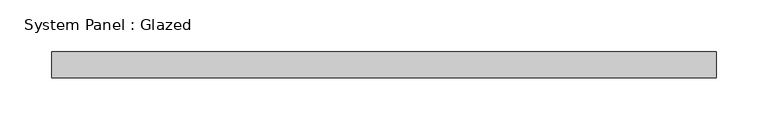
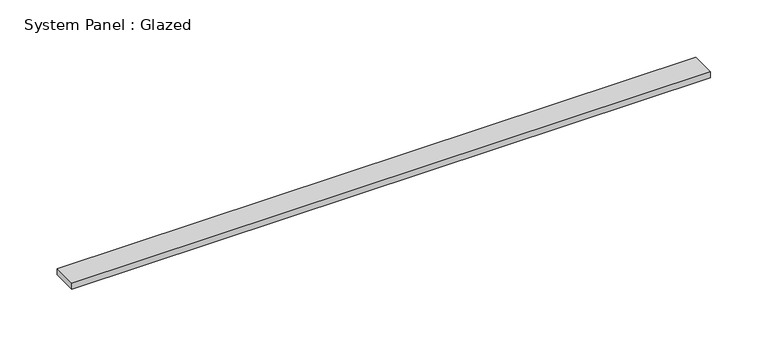
"""IFC4 building model written with IfcOpenShell, lengths in millimetres: plate geometry, System Panel : Glazed."""

from ifc_helpers import new_model, si_unit, origin, origin_with_axes, place, context, project, spatial, polyline, outline, extrude, source, transform, mapped, element, save


def system_panel_glazed_6aed1af6(model_context):
    return source(origin(), model_context, "Body", "SweptSolid", [
        extrude(outline(polyline([(321.7333333, 19.05), (-321.7333333, 19.05), (-321.7333333, 44.45), (321.7333333, 44.45), (321.7333333, 19.05)])), origin_with_axes(), (0.0, 0.0, 1.0), 6.35),
    ])


if __name__ == "__main__":
    model = new_model("IFC4")
    model_context = context("Model", 3, world=origin())
    ifc_project = project(units=[si_unit("LENGTHUNIT", "METRE", prefix="MILLI")], contexts=[model_context])
    site = spatial("IfcSite", under=ifc_project)
    building = spatial("IfcBuilding", under=site)
    placement = place(None, origin())
    system_panel_glazed_shape = system_panel_glazed_6aed1af6(model_context)
    element("IfcPlate", 1, ObjectType="System Panel : Glazed", at=placement, inside=building, context=model_context, shape_type="MappedRepresentation", body=[
        mapped(system_panel_glazed_shape, transform((0.0, 0.0, 0.0), x_axis=(1.0, 0.0, 0.0), y_axis=(0.0, 1.0, 0.0), z_axis=(0.0, 0.0, 1.0))),
    ])
    save(model, "model.ifc")

# Revit data of these elements
# Type "System Panel : Glazed"
#   Construction Type Id = "GSP4R"
#   Analytic Construction = "1/8 in Pilkington single glazing"
#   Visual Light Transmittance = 0.9
#   Solar Heat Gain Coefficient = 0.86
#   Heat Transfer Coefficient (U) = 1.18115 BTU/(h·ft²·°F)
#   Define Thermal Properties by = 1
# Element 1 (IfcPlate, "System Panel : Glazed")
#   Materials on its faces: "Glass"
# Materials
#   "Glass": class "Glass", colour RGB 0 128 192, transparency 0.75, Description = "Soda Lime Glass", Cost = 0
